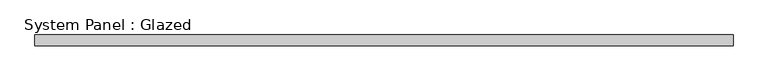
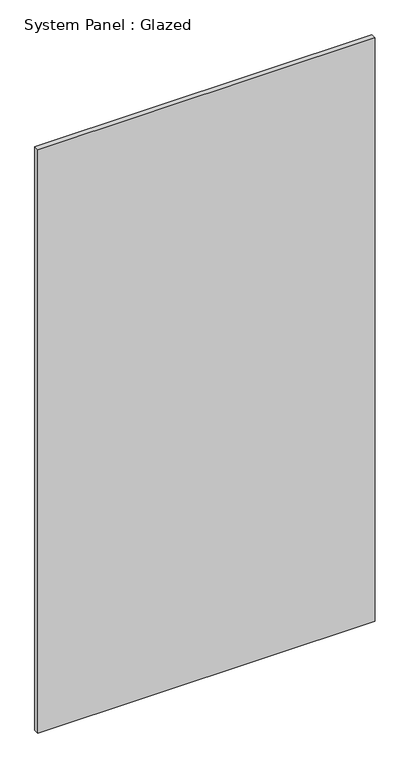
"""IFC4 building model written with IfcOpenShell, lengths in millimetres: plate geometry, System Panel : Glazed."""

from ifc_helpers import new_model, si_unit, origin, origin_with_axes, place, context, project, spatial, polyline, outline, extrude, source, transform, mapped, element, save


def system_panel_glazed_1e7c63f8(model_context):
    return source(origin(), model_context, "Body", "SweptSolid", [
        extrude(outline(polyline([(820.1879223, 24.5), (-820.1879223, 24.5), (-820.1879223, 49.5), (820.1879223, 49.5), (820.1879223, 24.5)])), origin_with_axes(), (0.0, 0.0, 1.0), 3000.0),
    ])


if __name__ == "__main__":
    model = new_model("IFC4")
    model_context = context("Model", 3, world=origin())
    ifc_project = project(units=[si_unit("LENGTHUNIT", "METRE", prefix="MILLI")], contexts=[model_context])
    site = spatial("IfcSite", under=ifc_project)
    building = spatial("IfcBuilding", under=site)
    placement = place(None, origin())
    system_panel_glazed_shape = system_panel_glazed_1e7c63f8(model_context)
    element("IfcPlate", 1, ObjectType="System Panel : Glazed", at=placement, inside=building, context=model_context, shape_type="MappedRepresentation", body=[
        mapped(system_panel_glazed_shape, transform((0.0, 0.0, 0.0), x_axis=(1.0, 0.0, 0.0), y_axis=(0.0, 1.0, 0.0), z_axis=(0.0, 0.0, 1.0))),
    ])
    save(model, "model.ifc")

# Revit data of these elements
# Type "System Panel : Glazed"
#   Keynote = "H11"
#   Construction Type Id = "GSP4R"
#   Analytic Construction = "1/8 in Pilkington single glazing"
#   Visual Light Transmittance = 0.9
#   Solar Heat Gain Coefficient = 0.86
#   Heat Transfer Coefficient (U) = 6.7069 W/(m²·K)
#   Define Thermal Properties by = 1
# Element 1 (IfcPlate, "System Panel : Glazed")
#   Materials on its faces: "Glass"
# Materials
#   "Glass": class "Glass", colour RGB 0 128 192, transparency 0.9, Description = "Soda Lime Glass", Cost = 0
